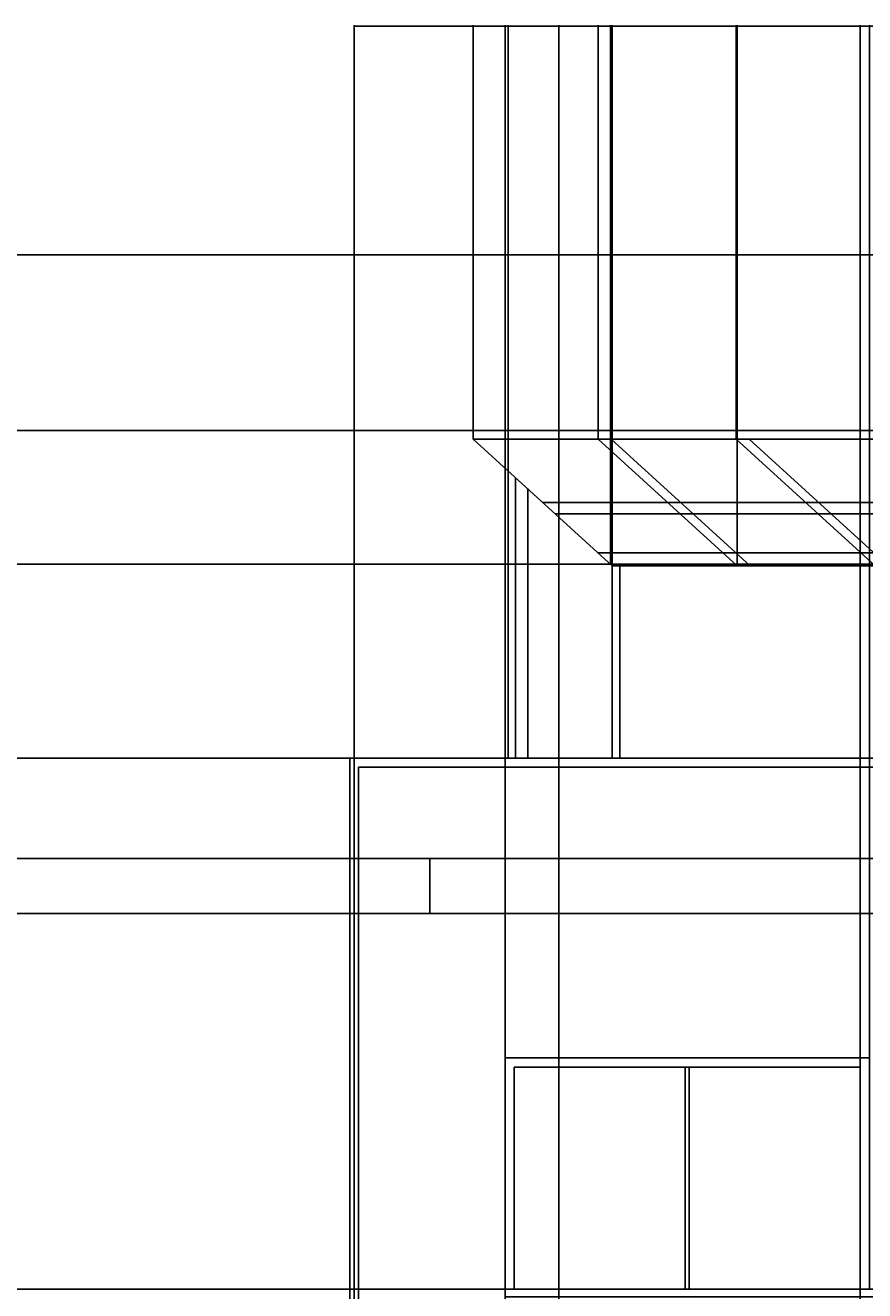
# Model space of a CAD drawing. Units: feet. Extents: x 2193 to 3502, y 890 to 1601.
# Tile 15 of 17: x 2848 to 3069, y 1268 to 1601. Entities that reach past the tile are written whole.
import ezdxf

# ---------------------------------------------------------------- set-up
doc = ezdxf.new("R2010")
doc.units = ezdxf.units.FT
doc.layers.add('A-ANNO-DIMS', color=2, linetype='Continuous', lineweight=18)
doc.layers.add('A-ELEV', color=7, linetype='Continuous', lineweight=25)
doc.styles.get("Standard").update_dxf_attribs({"font": 'arial.ttf'})
doc.dimstyles.get("Standard").update_dxf_attribs({"dimtxt": 0.18, "dimasz": 0.18, "dimexe": 0.18, "dimexo": 0.0625, "dimgap": 0.09, "dimtad": 0, "dimtih": 1, "dimtoh": 1, "dimdec": 0, "dimzin": 0, "dimdsep": 46, "dimlunit": 3, "dimtxsty": 'Standard', "dimcen": 0.09, "dimadec": 0, "dimazin": 0, "dimtfac": 1, "dimtdec": 0, "dimtofl": 0, "dimtmove": 0, "dimatfit": 3, "dimfxl": 1, "dimtolj": 1, "dimtzin": 0, "dimarcsym": 0})

# ---------------------------------------------------------------- blocks, each defined once
blk = doc.blocks.new('*D13')
at = {"layer": 'A-ANNO-DIMS', "color": 0, "lineweight": -2, "transparency": 16777216}
for p, q in [((2934.37, 950.89), (2934.37, 1601.47)), ((2934.55, 1601.29), (3186.64, 1601.29)), ((3439.51, 1601.29), (3187.43, 1601.29)), ((3439.69, 1541.11), (3439.69, 1601.47))]:
    blk.add_line(p, q, dxfattribs=at)
at = {"layer": 'A-ANNO-DIMS', "color": 0, "transparency": 16777216}
for points in [[(2934.55, 1601.32), (2934.55, 1601.26), (2934.37, 1601.29)], [(3439.51, 1601.32), (3439.51, 1601.26), (3439.69, 1601.29)]]:
    blk.add_solid(points, dxfattribs=at)
at = {"layer": 'Defpoints', "color": 0, "transparency": 16777216}
for p in [(3439.69, 1601.29), (3439.69, 1541.04), (2934.37, 950.82)]:
    blk.add_point(p, dxfattribs=at)
at = {"layer": 'A-ANNO-DIMS', "color": 0, "transparency": 16777216, "insert": (3187.03, 1601.29), "char_height": 0.18, "attachment_point": 5}
blk.add_mtext('\\A1;505.3', dxfattribs=at)
blk = doc.blocks.new('*D20')
at = {"layer": 'A-ANNO-DIMS', "color": 0, "lineweight": -2, "transparency": 16777216}
for p, q in [((2933.15, 1408.48), (2193.56, 1408.48)), ((2193.74, 1408.3), (2193.74, 1240.94)), ((2193.74, 1073.21), (2193.74, 1240.57)), ((2934.31, 1073.03), (2193.56, 1073.03))]:
    blk.add_line(p, q, dxfattribs=at)
at = {"layer": 'A-ANNO-DIMS', "color": 0, "transparency": 16777216}
for points in [[(2193.71, 1408.3), (2193.77, 1408.3), (2193.74, 1408.48)], [(2193.71, 1073.21), (2193.77, 1073.21), (2193.74, 1073.03)]]:
    blk.add_solid(points, dxfattribs=at)
at = {"layer": 'Defpoints', "color": 0, "transparency": 16777216}
for p in [(2193.74, 1408.48), (2933.21, 1408.48), (2934.37, 1073.03)]:
    blk.add_point(p, dxfattribs=at)
at = {"layer": 'A-ANNO-DIMS', "color": 0, "transparency": 16777216, "insert": (2193.74, 1240.76), "char_height": 0.18, "attachment_point": 5}
blk.add_mtext('\\A1;335.45', dxfattribs=at)
blk = doc.blocks.new('*D21')
at = {"layer": 'A-ANNO-DIMS', "color": 0, "lineweight": -2, "transparency": 16777216}
for p, q in [((2965.66, 1494.8), (2193.56, 1494.8)), ((2193.74, 1494.62), (2193.74, 1451.82)), ((2193.74, 1408.66), (2193.74, 1451.46)), ((2974.89, 1408.48), (2193.56, 1408.48))]:
    blk.add_line(p, q, dxfattribs=at)
at = {"layer": 'A-ANNO-DIMS', "color": 0, "transparency": 16777216}
for points in [[(2193.71, 1494.62), (2193.77, 1494.62), (2193.74, 1494.8)], [(2193.71, 1408.66), (2193.77, 1408.66), (2193.74, 1408.48)]]:
    blk.add_solid(points, dxfattribs=at)
at = {"layer": 'Defpoints', "color": 0, "transparency": 16777216}
for p in [(2193.74, 1494.8), (2965.72, 1494.8), (2974.95, 1408.48)]:
    blk.add_point(p, dxfattribs=at)
at = {"layer": 'A-ANNO-DIMS', "color": 0, "transparency": 16777216, "insert": (2193.74, 1451.64), "char_height": 0.18, "attachment_point": 5}
blk.add_mtext('\\A1;86.32', dxfattribs=at)
blk = doc.blocks.new('*D22')
at = {"layer": 'A-ANNO-DIMS', "color": 0, "lineweight": -2, "transparency": 16777216}
for p, q in [((2988.31, 1038.93), (2988.31, 1601.47)), ((2988.49, 1601.29), (3027.59, 1601.29)), ((3067.48, 1601.29), (3028.38, 1601.29)), ((3067.66, 1038.93), (3067.66, 1601.47))]:
    blk.add_line(p, q, dxfattribs=at)
at = {"layer": 'A-ANNO-DIMS', "color": 0, "transparency": 16777216}
for points in [[(2988.49, 1601.32), (2988.49, 1601.26), (2988.31, 1601.29)], [(3067.48, 1601.32), (3067.48, 1601.26), (3067.66, 1601.29)]]:
    blk.add_solid(points, dxfattribs=at)
at = {"layer": 'Defpoints', "color": 0, "transparency": 16777216}
for p in [(3067.66, 1601.29), (2988.31, 1038.87), (3067.66, 1038.87)]:
    blk.add_point(p, dxfattribs=at)
at = {"layer": 'A-ANNO-DIMS', "color": 0, "transparency": 16777216, "insert": (3027.98, 1601.29), "char_height": 0.18, "attachment_point": 5}
blk.add_mtext('\\A1;79.36', dxfattribs=at)
blk = doc.blocks.new('*D31')
at = {"layer": 'A-ANNO-DIMS', "color": 0, "lineweight": -2, "transparency": 16777216}
for p, q in [((2760.54, 1541.04), (3501.85, 1541.04)), ((3501.67, 1540.86), (3501.67, 1246.12)), ((3501.67, 951), (3501.67, 1245.75)), ((2762.27, 950.82), (3501.85, 950.82))]:
    blk.add_line(p, q, dxfattribs=at)
at = {"layer": 'A-ANNO-DIMS', "color": 0, "transparency": 16777216}
for points in [[(3501.64, 1540.86), (3501.7, 1540.86), (3501.67, 1541.04)], [(3501.64, 951), (3501.7, 951), (3501.67, 950.82)]]:
    blk.add_solid(points, dxfattribs=at)
at = {"layer": 'Defpoints', "color": 0, "transparency": 16777216}
for p in [(2760.47, 1541.04), (3501.67, 1541.04), (2762.2, 950.82)]:
    blk.add_point(p, dxfattribs=at)
at = {"layer": 'A-ANNO-DIMS', "color": 0, "transparency": 16777216, "insert": (3501.67, 1245.93), "char_height": 0.18, "attachment_point": 5}
blk.add_mtext('\\A1;590.2', dxfattribs=at)
blk = doc.blocks.new('*D36')
at = {"layer": 'A-ANNO-DIMS', "color": 0, "lineweight": -2, "transparency": 16777216}
for p, q in [((2974.05, 1268.66), (2193.56, 1268.66)), ((2193.74, 1268.48), (2193.74, 1200.71)), ((2193.74, 1132.57), (2193.74, 1200.34)), ((2980.65, 1132.39), (2193.56, 1132.39))]:
    blk.add_line(p, q, dxfattribs=at)
at = {"layer": 'A-ANNO-DIMS', "color": 0, "transparency": 16777216}
for points in [[(2193.71, 1268.48), (2193.77, 1268.48), (2193.74, 1268.66)], [(2193.71, 1132.57), (2193.77, 1132.57), (2193.74, 1132.39)]]:
    blk.add_solid(points, dxfattribs=at)
at = {"layer": 'Defpoints', "color": 0, "transparency": 16777216}
for p in [(2193.74, 1268.66), (2974.12, 1268.66), (2980.72, 1132.39)]:
    blk.add_point(p, dxfattribs=at)
at = {"layer": 'A-ANNO-DIMS', "color": 0, "transparency": 16777216, "insert": (2193.74, 1200.53), "char_height": 0.18, "attachment_point": 5}
blk.add_mtext('\\A1;136.27', dxfattribs=at)
blk = doc.blocks.new('*D37')
at = {"layer": 'A-ANNO-DIMS', "color": 0, "lineweight": -2, "transparency": 16777216}
for p, q in [((2974.05, 1367.57), (2193.56, 1367.57)), ((2193.74, 1367.39), (2193.74, 1318.3)), ((2193.74, 1268.84), (2193.74, 1317.93)), ((2974.05, 1268.66), (2193.56, 1268.66))]:
    blk.add_line(p, q, dxfattribs=at)
at = {"layer": 'A-ANNO-DIMS', "color": 0, "transparency": 16777216}
for points in [[(2193.71, 1367.39), (2193.77, 1367.39), (2193.74, 1367.57)], [(2193.71, 1268.84), (2193.77, 1268.84), (2193.74, 1268.66)]]:
    blk.add_solid(points, dxfattribs=at)
at = {"layer": 'Defpoints', "color": 0, "transparency": 16777216}
for p in [(2193.74, 1367.57), (2974.12, 1367.57), (2974.12, 1268.66)]:
    blk.add_point(p, dxfattribs=at)
at = {"layer": 'A-ANNO-DIMS', "color": 0, "transparency": 16777216, "insert": (2193.74, 1318.12), "char_height": 0.18, "attachment_point": 5}
blk.add_mtext('\\A1;98.91', dxfattribs=at)
blk = doc.blocks.new('*D38')
at = {"layer": 'A-ANNO-DIMS', "color": 0, "lineweight": -2, "transparency": 16777216}
for p, q in [((2954.2, 1382.08), (2193.56, 1382.08)), ((2193.74, 1381.9), (2193.74, 1375.01)), ((2193.74, 1367.75), (2193.74, 1374.64)), ((2954.2, 1367.57), (2193.56, 1367.57))]:
    blk.add_line(p, q, dxfattribs=at)
at = {"layer": 'A-ANNO-DIMS', "color": 0, "transparency": 16777216}
for points in [[(2193.71, 1381.9), (2193.77, 1381.9), (2193.74, 1382.08)], [(2193.71, 1367.75), (2193.77, 1367.75), (2193.74, 1367.57)]]:
    blk.add_solid(points, dxfattribs=at)
at = {"layer": 'Defpoints', "color": 0, "transparency": 16777216}
for p in [(2193.74, 1382.08), (2954.26, 1382.08), (2954.26, 1367.57)]:
    blk.add_point(p, dxfattribs=at)
at = {"layer": 'A-ANNO-DIMS', "color": 0, "transparency": 16777216, "insert": (2193.74, 1374.83), "char_height": 0.18, "attachment_point": 5}
blk.add_mtext('\\A1;14.502', dxfattribs=at)
blk = doc.blocks.new('*D39')
at = {"layer": 'A-ANNO-DIMS', "color": 0, "lineweight": -2, "transparency": 16777216}
for p, q in [((2933.15, 1408.48), (2193.56, 1408.48)), ((2193.74, 1408.3), (2193.74, 1395.46)), ((2193.74, 1382.26), (2193.74, 1395.1)), ((2954.2, 1382.08), (2193.56, 1382.08))]:
    blk.add_line(p, q, dxfattribs=at)
at = {"layer": 'A-ANNO-DIMS', "color": 0, "transparency": 16777216}
for points in [[(2193.71, 1408.3), (2193.77, 1408.3), (2193.74, 1408.48)], [(2193.71, 1382.26), (2193.77, 1382.26), (2193.74, 1382.08)]]:
    blk.add_solid(points, dxfattribs=at)
at = {"layer": 'Defpoints', "color": 0, "transparency": 16777216}
for p in [(2193.74, 1408.48), (2933.21, 1408.48), (2954.26, 1382.08)]:
    blk.add_point(p, dxfattribs=at)
at = {"layer": 'A-ANNO-DIMS', "color": 0, "transparency": 16777216, "insert": (2193.74, 1395.28), "char_height": 0.18, "attachment_point": 5}
blk.add_mtext('\\A1;26.405', dxfattribs=at)
blk = doc.blocks.new('*D48')
at = {"layer": 'A-ANNO-DIMS', "color": 0, "lineweight": -2, "transparency": 16777216}
for p, q in [((2965.72, 1494.87), (2965.72, 1601.47)), ((2965.9, 1601.29), (3123.44, 1601.29)), ((3281.9, 1601.29), (3124.36, 1601.29)), ((3282.08, 1494.87), (3282.08, 1601.47))]:
    blk.add_line(p, q, dxfattribs=at)
at = {"layer": 'A-ANNO-DIMS', "color": 0, "transparency": 16777216}
for points in [[(2965.9, 1601.32), (2965.9, 1601.26), (2965.72, 1601.29)], [(3281.9, 1601.32), (3281.9, 1601.26), (3282.08, 1601.29)]]:
    blk.add_solid(points, dxfattribs=at)
at = {"layer": 'Defpoints', "color": 0, "transparency": 16777216}
for p in [(3282.08, 1601.29), (2965.72, 1494.8), (3282.08, 1494.8)]:
    blk.add_point(p, dxfattribs=at)
at = {"layer": 'A-ANNO-DIMS', "color": 0, "transparency": 16777216, "insert": (3123.9, 1601.29), "char_height": 0.18, "attachment_point": 5}
blk.add_mtext('\\A1;316.36', dxfattribs=at)
blk = doc.blocks.new('*D49')
at = {"layer": 'A-ANNO-DIMS', "color": 0, "lineweight": -2, "transparency": 16777216}
for p, q in [((2965.72, 1492.58), (2965.72, 1601.47)), ((2965.9, 1601.29), (2983.34, 1601.29)), ((3001.71, 1601.29), (2984.27, 1601.29)), ((3001.89, 1459.67), (3001.89, 1601.47))]:
    blk.add_line(p, q, dxfattribs=at)
at = {"layer": 'A-ANNO-DIMS', "color": 0, "transparency": 16777216}
for points in [[(2965.9, 1601.32), (2965.9, 1601.26), (2965.72, 1601.29)], [(3001.71, 1601.32), (3001.71, 1601.26), (3001.89, 1601.29)]]:
    blk.add_solid(points, dxfattribs=at)
at = {"layer": 'Defpoints', "color": 0, "transparency": 16777216}
for p in [(3001.89, 1601.29), (2965.72, 1492.51), (3001.89, 1459.6)]:
    blk.add_point(p, dxfattribs=at)
at = {"layer": 'A-ANNO-DIMS', "color": 0, "transparency": 16777216, "insert": (2983.81, 1601.29), "char_height": 0.18, "attachment_point": 5}
blk.add_mtext('\\A1;36.175', dxfattribs=at)
blk = doc.blocks.new('*D51')
at = {"layer": 'A-ANNO-DIMS', "color": 0, "lineweight": -2, "transparency": 16777216}
for p, q in [((2965.78, 1492.51), (3501.85, 1492.51)), ((3501.67, 1492.33), (3501.67, 1476.24)), ((3501.67, 1459.78), (3501.67, 1475.88)), ((3001.96, 1459.6), (3501.85, 1459.6))]:
    blk.add_line(p, q, dxfattribs=at)
at = {"layer": 'A-ANNO-DIMS', "color": 0, "transparency": 16777216}
for points in [[(3501.64, 1492.33), (3501.7, 1492.33), (3501.67, 1492.51)], [(3501.64, 1459.78), (3501.7, 1459.78), (3501.67, 1459.6)]]:
    blk.add_solid(points, dxfattribs=at)
at = {"layer": 'Defpoints', "color": 0, "transparency": 16777216}
for p in [(2965.72, 1492.51), (3501.67, 1492.51), (3001.89, 1459.6)]:
    blk.add_point(p, dxfattribs=at)
at = {"layer": 'A-ANNO-DIMS', "color": 0, "transparency": 16777216, "insert": (3501.67, 1476.06), "char_height": 0.18, "attachment_point": 5}
blk.add_mtext('\\A1;32.91', dxfattribs=at)
blk = doc.blocks.new('*D52')
at = {"layer": 'A-ANNO-DIMS', "color": 0, "lineweight": -2, "transparency": 16777216}
for p, q in [((2998.66, 1492.58), (2998.66, 1601.47)), ((2998.84, 1601.29), (3016.37, 1601.29)), ((3034.83, 1601.29), (3017.3, 1601.29)), ((3035.01, 1492.58), (3035.01, 1601.47))]:
    blk.add_line(p, q, dxfattribs=at)
at = {"layer": 'A-ANNO-DIMS', "color": 0, "transparency": 16777216}
for points in [[(2998.84, 1601.32), (2998.84, 1601.26), (2998.66, 1601.29)], [(3034.83, 1601.32), (3034.83, 1601.26), (3035.01, 1601.29)]]:
    blk.add_solid(points, dxfattribs=at)
at = {"layer": 'Defpoints', "color": 0, "transparency": 16777216}
for p in [(3035.01, 1601.29), (2998.66, 1492.51), (3035.01, 1492.51)]:
    blk.add_point(p, dxfattribs=at)
at = {"layer": 'A-ANNO-DIMS', "color": 0, "transparency": 16777216, "insert": (3016.83, 1601.29), "char_height": 0.18, "attachment_point": 5}
blk.add_mtext('\\A1;36.355', dxfattribs=at)
blk = doc.blocks.new('*D53')
at = {"layer": 'A-ANNO-DIMS', "color": 0, "lineweight": -2, "transparency": 16777216}
for p, q in [((2974.95, 1408.54), (2974.95, 1601.47)), ((2975.13, 1601.29), (2988.27, 1601.29)), ((3002.2, 1601.29), (2989.06, 1601.29)), ((3002.38, 1408.54), (3002.38, 1601.47))]:
    blk.add_line(p, q, dxfattribs=at)
at = {"layer": 'A-ANNO-DIMS', "color": 0, "transparency": 16777216}
for points in [[(2975.13, 1601.32), (2975.13, 1601.26), (2974.95, 1601.29)], [(3002.2, 1601.32), (3002.2, 1601.26), (3002.38, 1601.29)]]:
    blk.add_solid(points, dxfattribs=at)
at = {"layer": 'Defpoints', "color": 0, "transparency": 16777216}
for p in [(3002.38, 1601.29), (2974.95, 1408.48), (3002.38, 1408.48)]:
    blk.add_point(p, dxfattribs=at)
at = {"layer": 'A-ANNO-DIMS', "color": 0, "transparency": 16777216, "insert": (2988.67, 1601.29), "char_height": 0.18, "attachment_point": 5}
blk.add_mtext('\\A1;27.43', dxfattribs=at)
blk = doc.blocks.new('*D54')
at = {"layer": 'A-ANNO-DIMS', "color": 0, "lineweight": -2, "transparency": 16777216}
for p, q in [((3002.38, 1408.54), (3002.38, 1601.47)), ((3002.56, 1601.29), (3043.2, 1601.29)), ((3084.62, 1601.29), (3043.99, 1601.29)), ((3084.8, 1408.54), (3084.8, 1601.47))]:
    blk.add_line(p, q, dxfattribs=at)
at = {"layer": 'A-ANNO-DIMS', "color": 0, "transparency": 16777216}
for points in [[(3002.56, 1601.32), (3002.56, 1601.26), (3002.38, 1601.29)], [(3084.62, 1601.32), (3084.62, 1601.26), (3084.8, 1601.29)]]:
    blk.add_solid(points, dxfattribs=at)
at = {"layer": 'Defpoints', "color": 0, "transparency": 16777216}
for p in [(3084.8, 1601.29), (3002.38, 1408.48), (3084.8, 1408.48)]:
    blk.add_point(p, dxfattribs=at)
at = {"layer": 'A-ANNO-DIMS', "color": 0, "transparency": 16777216, "insert": (3043.59, 1601.29), "char_height": 0.18, "attachment_point": 5}
blk.add_mtext('\\A1;82.42', dxfattribs=at)
blk = doc.blocks.new('*D58')
at = {"layer": 'A-ANNO-DIMS', "color": 0, "lineweight": -2, "transparency": 16777216}
for p, q in [((3001.83, 1459.6), (2193.56, 1459.6)), ((2193.74, 1459.42), (2193.74, 1434.22)), ((2193.74, 1408.66), (2193.74, 1433.86)), ((2974.89, 1408.48), (2193.56, 1408.48))]:
    blk.add_line(p, q, dxfattribs=at)
at = {"layer": 'A-ANNO-DIMS', "color": 0, "transparency": 16777216}
for points in [[(2193.71, 1459.42), (2193.77, 1459.42), (2193.74, 1459.6)], [(2193.71, 1408.66), (2193.77, 1408.66), (2193.74, 1408.48)]]:
    blk.add_solid(points, dxfattribs=at)
at = {"layer": 'Defpoints', "color": 0, "transparency": 16777216}
for p in [(2193.74, 1459.6), (3001.89, 1459.6), (2974.95, 1408.48)]:
    blk.add_point(p, dxfattribs=at)
at = {"layer": 'A-ANNO-DIMS', "color": 0, "transparency": 16777216, "insert": (2193.74, 1434.04), "char_height": 0.18, "attachment_point": 5}
blk.add_mtext('\\A1;51.12', dxfattribs=at)
blk = doc.blocks.new('*D59')
at = {"layer": 'A-ANNO-DIMS', "color": 0, "lineweight": -2, "transparency": 16777216}
for p, q in [((2974.12, 1329.64), (2974.12, 1601.47)), ((2974.3, 1601.29), (3021.89, 1601.29)), ((3069.93, 1601.29), (3022.33, 1601.29)), ((3070.11, 1329.64), (3070.11, 1601.47))]:
    blk.add_line(p, q, dxfattribs=at)
at = {"layer": 'A-ANNO-DIMS', "color": 0, "transparency": 16777216}
for points in [[(2974.3, 1601.32), (2974.3, 1601.26), (2974.12, 1601.29)], [(3069.93, 1601.32), (3069.93, 1601.26), (3070.11, 1601.29)]]:
    blk.add_solid(points, dxfattribs=at)
at = {"layer": 'Defpoints', "color": 0, "transparency": 16777216}
for p in [(3070.11, 1601.29), (2974.12, 1329.58), (3070.11, 1329.58)]:
    blk.add_point(p, dxfattribs=at)
at = {"layer": 'A-ANNO-DIMS', "color": 0, "transparency": 16777216, "insert": (3022.11, 1601.29), "char_height": 0.18, "attachment_point": 5}
blk.add_mtext('\\A1;96', dxfattribs=at)
blk = doc.blocks.new('*D127')
at = {"layer": 'A-ANNO-DIMS', "color": 0, "lineweight": -2, "transparency": 16777216}
for p, q in [((2965.72, 1492.58), (2965.72, 1601.47)), ((2965.9, 1601.29), (2981.72, 1601.29)), ((2998.48, 1601.29), (2982.65, 1601.29)), ((2998.66, 1492.58), (2998.66, 1601.47))]:
    blk.add_line(p, q, dxfattribs=at)
at = {"layer": 'A-ANNO-DIMS', "color": 0, "transparency": 16777216}
for points in [[(2965.9, 1601.32), (2965.9, 1601.26), (2965.72, 1601.29)], [(2998.48, 1601.32), (2998.48, 1601.26), (2998.66, 1601.29)]]:
    blk.add_solid(points, dxfattribs=at)
at = {"layer": 'Defpoints', "color": 0, "transparency": 16777216}
for p in [(2998.66, 1601.29), (2965.72, 1492.51), (2998.66, 1492.51)]:
    blk.add_point(p, dxfattribs=at)
at = {"layer": 'A-ANNO-DIMS', "color": 0, "transparency": 16777216, "insert": (2982.19, 1601.29), "char_height": 0.18, "attachment_point": 5}
blk.add_mtext('\\A1;32.936', dxfattribs=at)
blk = doc.blocks.new('*D128')
at = {"layer": 'A-ANNO-DIMS', "color": 0, "lineweight": -2, "transparency": 16777216}
for p, q in [((2998.66, 1492.58), (2998.66, 1601.47)), ((2998.84, 1601.29), (3016.59, 1601.29)), ((3035.14, 1601.29), (3017.38, 1601.29)), ((3035.32, 1459.22), (3035.32, 1601.47))]:
    blk.add_line(p, q, dxfattribs=at)
at = {"layer": 'A-ANNO-DIMS', "color": 0, "transparency": 16777216}
for points in [[(2998.84, 1601.32), (2998.84, 1601.26), (2998.66, 1601.29)], [(3035.14, 1601.32), (3035.14, 1601.26), (3035.32, 1601.29)]]:
    blk.add_solid(points, dxfattribs=at)
at = {"layer": 'Defpoints', "color": 0, "transparency": 16777216}
for p in [(3035.32, 1601.29), (2998.66, 1492.51), (3035.32, 1459.16)]:
    blk.add_point(p, dxfattribs=at)
at = {"layer": 'A-ANNO-DIMS', "color": 0, "transparency": 16777216, "insert": (3016.99, 1601.29), "char_height": 0.18, "attachment_point": 5}
blk.add_mtext('\\A1;36.66', dxfattribs=at)

msp = doc.modelspace()

# ---------------------------------------------------------------- linework, layer by layer
at = {"layer": 'A-ELEV'}
for p, q in [((2965.7197, 1492.5146), (3002.3827, 1459.1592)), ((2998.6559, 1492.5146), (3035.3189, 1459.1592)), ((3002.0745, 1492.5146), (3038.7375, 1459.1592)), ((3035.0107, 1492.5146), (3071.6737, 1459.1592)), ((3038.4293, 1492.5146), (3075.0923, 1459.1592)), ((2980.0933, 1479.4377), (2980.0933, 1408.4814)), ((3270.9554, 1475.8561), (2984.0301, 1475.8561)), ((3268.9492, 1472.8525), (2987.3316, 1472.8525)), ((3262.1063, 1462.6071), (2998.5929, 1462.6071)), ((3260.1002, 1459.6035), (3001.8944, 1459.6035)), ((3002.3827, 1459.1592), (3259.8035, 1459.1592))]:
    msp.add_line(p, q, dxfattribs=at)
for points in [[(3282.0816, 1494.8043), (2965.7197, 1494.8043), (2965.7197, 1492.5146), (3282.0816, 1492.5146)], [(3002.3827, 1459.1592), (3004.3888, 1459.1592), (3004.3888, 1408.4814), (3002.3827, 1408.4814)], [(2974.116, 1268.6599), (3070.1101, 1268.6599), (3070.1101, 1329.5765), (2974.116, 1329.5765)], [(3021.5849, 1327.1314), (3022.6412, 1327.1314), (3022.6412, 1268.6599), (3021.5849, 1268.6599)], [(2974.116, 1266.7092), (3147.5022, 1266.7092), (3147.5022, 1268.6599), (2974.116, 1268.6599)]]:
    msp.add_lwpolyline(points, close=True, dxfattribs=at)
for points in [[(2974.9536, 1408.4814), (2974.9536, 1484.1138)], [(2976.9105, 1482.3334), (2976.9105, 1408.4814)], [(2934.3742, 1089.3627), (2933.2085, 1089.3627), (2933.2085, 1408.4814), (2934.3742, 1408.4814)], [(3215.7583, 1408.4814), (2934.3742, 1408.4814)], [(2934.3742, 1089.3627), (2935.5399, 1089.3627), (2935.5399, 1406.15)], [(2935.5399, 1406.15), (3215.7583, 1406.15), (3215.7583, 1407.3157)], [(3425.1877, 1367.5739), (2954.2649, 1367.5739), (2954.2649, 1382.0763), (3439.6901, 1382.0763), (3439.6901, 1367.5739)], [(2934.3742, 1089.3627), (2934.3742, 1073.031), (2974.116, 1073.031), (2974.116, 1367.5739)], [(2974.116, 1367.5739), (3215.7583, 1367.5739)], [(3067.665, 1268.6599), (3067.665, 1327.1314), (2976.5611, 1327.1314), (2976.5611, 1268.6599)]]:
    msp.add_lwpolyline(points, dxfattribs=at)

# ---------------------------------------------------------------- dimensions: what is measured, and where the dimension line sits
at = {"layer": 'A-ANNO-DIMS'}
for base, p1, p2, override, picture, middle in [((3439.6901, 1601.2941), (2934.3742, 950.8228), (3439.6901, 1541.0441), {"dimdec": 1, "dimlfac": 1, "dimrnd": 0, "dimzin": 0, "dimdsep": 46, "dimlunit": 2}, '*D13', (3187.0321, 1601.2941)), ((3282.0816, 1601.2941), (2965.7197, 1494.8043), (3282.0816, 1494.8043), {"dimdec": 2, "dimlfac": 1, "dimrnd": 0, "dimzin": 0, "dimdsep": 46, "dimlunit": 2}, '*D48', (3123.9006, 1601.2941)), ((3001.8944, 1601.2941), (2965.7197, 1492.5146), (3001.8944, 1459.6035), {"dimdec": 3, "dimlfac": 1, "dimrnd": 0, "dimzin": 0, "dimdsep": 46, "dimlunit": 2}, '*D49', (2983.807, 1601.2941)), ((2998.6559, 1601.2941), (2965.7197, 1492.5146), (2998.6559, 1492.5146), {"dimdec": 3, "dimlfac": 1, "dimrnd": 0, "dimzin": 0, "dimdsep": 46, "dimlunit": 2}, '*D127', (2982.1878, 1601.2941)), ((3070.1101, 1601.2941), (2974.116, 1329.5765), (3070.1101, 1329.5765), {"dimdec": 0, "dimlfac": 1, "dimrnd": 0, "dimzin": 0, "dimdsep": 46, "dimlunit": 2}, '*D59', (3022.113, 1601.2941)), ((3002.3827, 1601.2941), (2974.9536, 1408.4814), (3002.3827, 1408.4814), {"dimdec": 2, "dimlfac": 1, "dimrnd": 0, "dimzin": 0, "dimdsep": 46, "dimlunit": 2}, '*D53', (2988.6681, 1601.2941)), ((3067.665, 1601.2941), (2988.305, 1038.8658), (3067.665, 1038.8658), {"dimdec": 2, "dimlfac": 1, "dimrnd": 0, "dimzin": 0, "dimdsep": 46, "dimlunit": 2}, '*D22', (3027.985, 1601.2941)), ((3035.0107, 1601.2941), (2998.6559, 1492.5146), (3035.0107, 1492.5146), {"dimdec": 3, "dimlfac": 1, "dimrnd": 0, "dimzin": 0, "dimdsep": 46, "dimlunit": 2}, '*D52', (3016.8333, 1601.2941)), ((3035.3189, 1601.2941), (2998.6559, 1492.5146), (3035.3189, 1459.1592), {"dimdec": 2, "dimlfac": 1, "dimrnd": 0, "dimzin": 0, "dimdsep": 46, "dimlunit": 2}, '*D128', (3016.9874, 1601.2941)), ((3084.8031, 1601.2941), (3002.3827, 1408.4814), (3084.8031, 1408.4814), {"dimdec": 2, "dimlfac": 1, "dimrnd": 0, "dimzin": 0, "dimdsep": 46, "dimlunit": 2}, '*D54', (3043.5929, 1601.2941))]:
    dim = msp.add_linear_dim(base=base, p1=p1, p2=p2, dimstyle='Standard', override=override, dxfattribs=at)
    dim.commit()
    dim.dimension.update_dxf_attribs({"geometry": picture, "text_midpoint": middle})
for base, p1, p2, override, picture, middle in [((3501.6716, 1541.0441), (2762.2048, 950.8228), (2760.4733, 1541.0441), {"dimdec": 1, "dimlfac": 1, "dimrnd": 0, "dimzin": 0, "dimdsep": 46, "dimlunit": 2}, '*D31', (3501.6716, 1245.9334)), ((2193.7417, 1494.8043), (2974.9536, 1408.4814), (2965.7197, 1494.8043), {"dimdec": 2, "dimlfac": 1, "dimrnd": 0, "dimzin": 0, "dimdsep": 46, "dimlunit": 2}, '*D21', (2193.7417, 1451.6429)), ((3501.6716, 1492.5146), (3001.8944, 1459.6035), (2965.7197, 1492.5146), {"dimdec": 2, "dimlfac": 1, "dimrnd": 0, "dimzin": 0, "dimdsep": 46, "dimlunit": 2}, '*D51', (3501.6716, 1476.0591)), ((2193.7417, 1459.6035), (2974.9536, 1408.4814), (3001.8944, 1459.6035), {"dimdec": 2, "dimlfac": 1, "dimrnd": 0, "dimzin": 0, "dimdsep": 46, "dimlunit": 2}, '*D58', (2193.7417, 1434.0425)), ((2193.7417, 1408.4814), (2934.3742, 1073.031), (2933.2085, 1408.4814), {"dimdec": 2, "dimlfac": 1, "dimrnd": 0, "dimzin": 0, "dimdsep": 46, "dimlunit": 2}, '*D20', (2193.7417, 1240.7562)), ((2193.7417, 1408.4814), (2954.2649, 1382.0763), (2933.2085, 1408.4814), {"dimdec": 3, "dimlfac": 1, "dimrnd": 0, "dimzin": 0, "dimdsep": 46, "dimlunit": 2}, '*D39', (2193.7417, 1395.2789)), ((2193.7417, 1382.0763), (2954.2649, 1367.5739), (2954.2649, 1382.0763), {"dimdec": 3, "dimlfac": 1, "dimrnd": 0, "dimzin": 0, "dimdsep": 46, "dimlunit": 2}, '*D38', (2193.7417, 1374.8251)), ((2193.7417, 1367.5739), (2974.116, 1268.6599), (2974.116, 1367.5739), {"dimdec": 2, "dimlfac": 1, "dimrnd": 0, "dimzin": 0, "dimdsep": 46, "dimlunit": 2}, '*D37', (2193.7417, 1318.1169)), ((2193.7417, 1268.6599), (2980.7151, 1132.3937), (2974.116, 1268.6599), {"dimdec": 2, "dimlfac": 1, "dimrnd": 0, "dimzin": 0, "dimdsep": 46, "dimlunit": 2}, '*D36', (2193.7417, 1200.5268))]:
    dim = msp.add_linear_dim(base=base, p1=p1, p2=p2, angle=90, dimstyle='Standard', override=override, dxfattribs=at)
    dim.commit()
    dim.dimension.update_dxf_attribs({"geometry": picture, "text_midpoint": middle})

doc.saveas('drawing.dxf')
